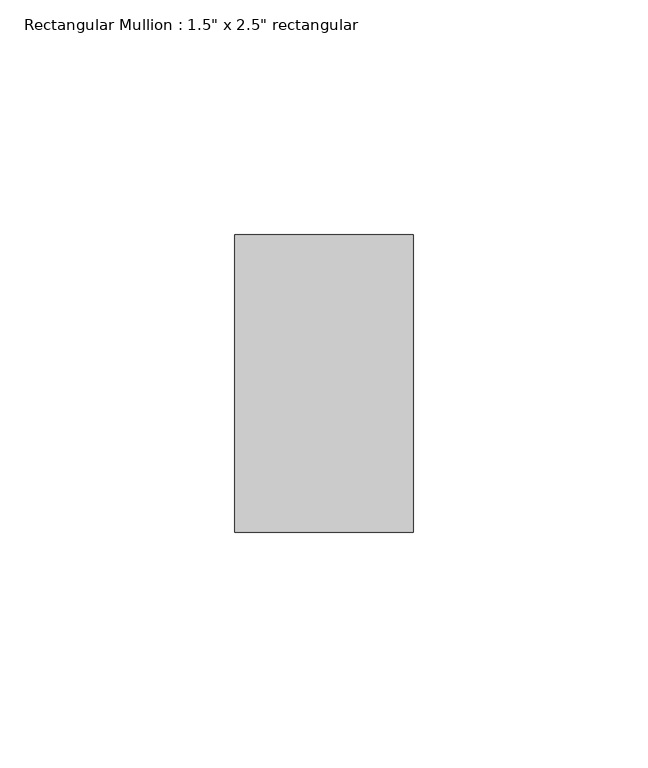
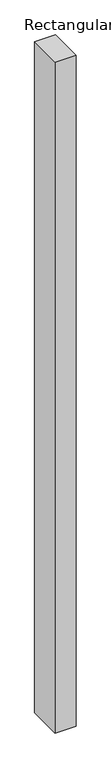
"""IFC4 building model written with IfcOpenShell, lengths in millimetres: member geometry."""

from ifc_helpers import new_model, si_unit, frame, origin, place, context, project, spatial, polyline, outline, extrude, source, transform, mapped, element, save


def member_03258ea9(model_context):
    return source(origin(), model_context, "Body", "SweptSolid", [
        extrude(outline(polyline([(19.05, 31.75), (19.05, -31.75), (-19.05, -31.75), (-19.05, 31.75), (19.05, 31.75)])), frame((0.0, 0.0, -1282.7), z_axis=(0.0, 0.0, 1.0), x_axis=(1.0, 0.0, 0.0)), (0.0, 0.0, 1.0), 1282.7),
    ])


if __name__ == "__main__":
    model = new_model("IFC4")
    model_context = context("Model", 3, world=origin())
    ifc_project = project(units=[si_unit("LENGTHUNIT", "METRE", prefix="MILLI")], contexts=[model_context])
    site = spatial("IfcSite", under=ifc_project)
    building = spatial("IfcBuilding", under=site)
    placement = place(None, origin())
    member_shape = member_03258ea9(model_context)
    element("IfcMember", 1, ObjectType="Rectangular Mullion : 1.5\" x 2.5\" rectangular", at=placement, inside=building, context=model_context, shape_type="MappedRepresentation", body=[
        mapped(member_shape, transform((0.0, 0.0, 0.0), x_axis=(1.0, 0.0, 0.0), y_axis=(0.0, 1.0, 0.0), z_axis=(0.0, 0.0, 1.0))),
    ])
    save(model, "model.ifc")

# Revit data of these elements
# Type "Rectangular Mullion : 1.5\" x 2.5\" rectangular"
#   built-in parameter 1007304 = 0.208333 (stored number, unit not read)
#   built-in parameter 1007301 = 0.0625 (stored number, unit not read)
#   built-in parameter 1007300 = 0.0625 (stored number, unit not read)
# Element 1 (IfcMember, "Rectangular Mullion : 1.5\" x 2.5\" rectangular")
#   Materials on its faces: "Damp-proofing"
# Materials
#   "Damp-proofing": class "Generic", colour RGB 127 127 127, transparency 0, Description = "Damp-proofing", Cost = 0
